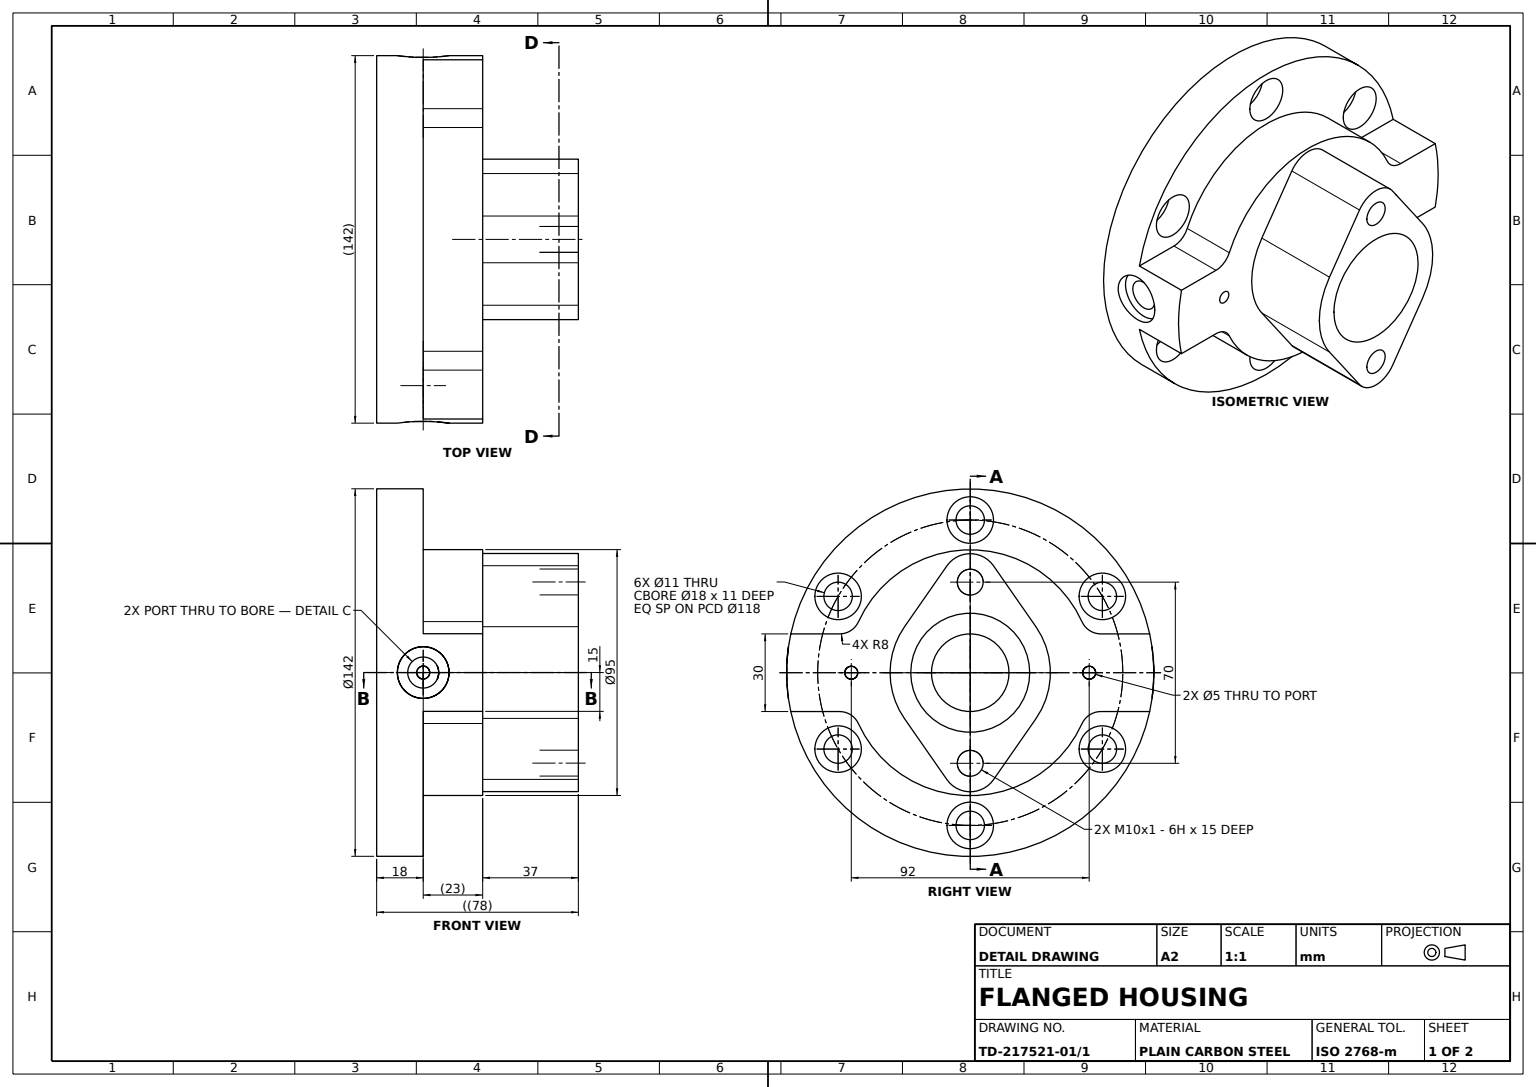
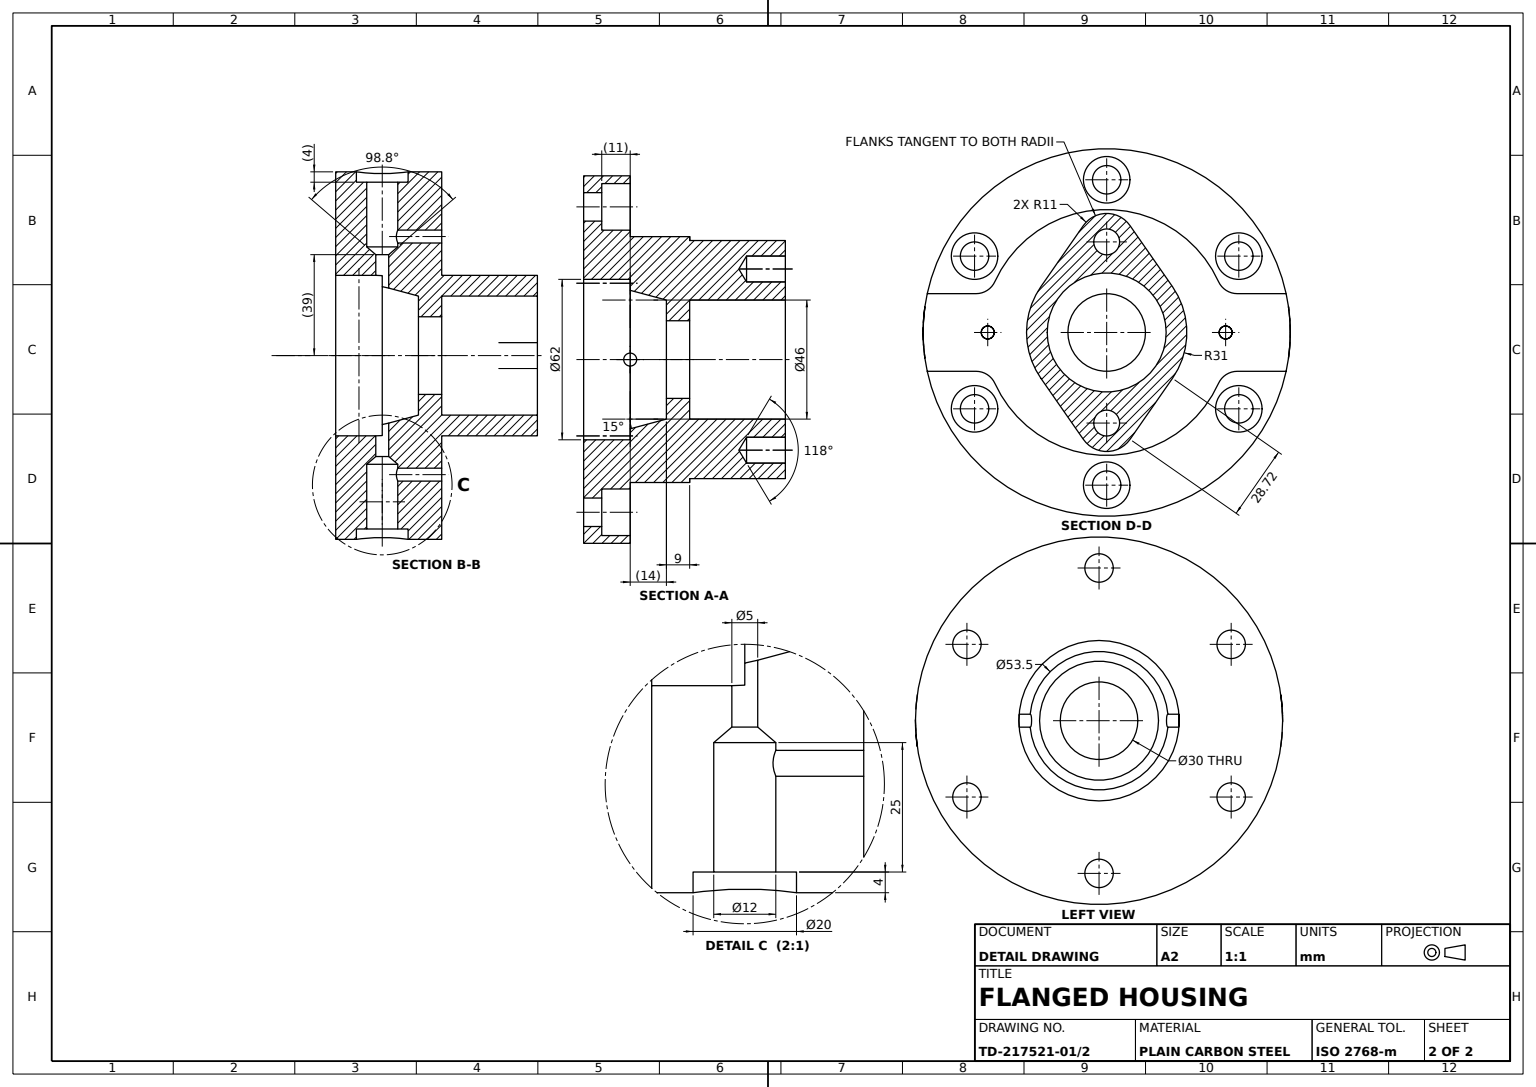
SolidWorks part; units mm, degrees
material "Plain Carbon Steel"
ref_plane "Front Plane" through (0, 0, 0) normal (0, 0, 1) x (1, 0, 0)
ref_plane "Top Plane" through (0, 0, 0) normal (0, 1, 0) x (1, 0, 0)
ref_plane "Right Plane" through (0, 0, 0) normal (1, 0, 0) x (0, 0, -1)
sketch "Base Flange Sketch" plane through (0, 0, 0) normal (0, 0, 1) x (1, 0, 0)
  circle A0 centre (0, 0) radius 71
  dimension "D1" = 142
extrude "Base Flange Ø142" add sketch "Base Flange Sketch" along normal blind 18
sketch "Middle Boss Sketch" plane through (0, 0, 0) normal (0, 0, -1) x (-1, 0, 0)
  line L0 (-81.5219, 0) -> (75.8672, 0) construction
  line L1 (50.5099, 15) -> (69.3974, 15)
  line L2 (50.5099, -15) -> (69.3974, -15)
  line L3 (0, 108.8072) -> (0, -83.8209) construction
  line L4 (-50.5099, -15) -> (-69.3974, -15)
  line L5 (-50.5099, 15) -> (-69.3974, 15)
  arc A0 (43.2292, 19.6847) -> (-43.2292, 19.6847) centre (0, 0) ccw
  arc A1 (69.3974, -15) -> (69.3974, 15) centre (0, 0) ccw
  circle A5 centre (0, 0) radius 71 construction
  arc A6 (-69.3974, 15) -> (-69.3974, -15) centre (0, 0) ccw
  arc A7 (-43.2292, -19.6847) -> (43.2292, -19.6847) centre (0, 0) ccw
  arc A8 (50.5099, -15) -> (43.2292, -19.6847) centre (50.5099, -23) ccw
  arc A9 (50.5099, 15) -> (43.2292, 19.6847) centre (50.5099, 23) cw
  arc A10 (-43.2292, 19.6847) -> (-50.5099, 15) centre (-50.5099, 23) cw
  arc A11 (-50.5099, -15) -> (-43.2292, -19.6847) centre (-50.5099, -23) cw
  point P17 (45.0694, -15)
  point P20 (45.0694, 15)
  point P23 (-45.0694, 15)
  point P26 (-45.0694, -15)
  dimension "D1" = 95
  dimension "D3" = 8
  dimension "D2" = 15
extrude "Middle Boss" add sketch "Middle Boss Sketch" along normal blind 23
sketch "Oval Flange Sketch" plane through (0, 0, -23) normal (0, 0, -1) x (-1, 0, 0)
  line L0 (0, 31.4693) -> (0, -35) construction
  line L1 (-58.0152, 0) -> (50.3973, 0) construction
  line L2 (-9.0272, 41.2857) -> (-25.4402, 17.7143)
  line L3 (9.0272, 41.2857) -> (25.4402, 17.7143)
  line L4 (9.0272, -41.2857) -> (25.4402, -17.7143)
  line L5 (-9.0272, -41.2857) -> (-25.4402, -17.7143)
  circle A1 centre (0, 0) radius 23
  arc A2 (-25.4402, 17.7143) -> (-25.4402, -17.7143) centre (0, 0) ccw
  arc A6 (9.0272, -41.2857) -> (-9.0272, -41.2857) centre (0, -35) cw
  arc A7 (25.4402, -17.7143) -> (25.4402, 17.7143) centre (0, 0) ccw
  arc A8 (9.0272, 41.2857) -> (-9.0272, 41.2857) centre (0, 35) ccw
  dimension "D1" = 62
  dimension "D2" = 46
  dimension "D3" = 70
  dimension "D5" = 28.7228
  dimension "D6" = 11
extrude "Oval Top Flange" add sketch "Oval Flange Sketch" along normal blind 37
sketch "Bolt Hole Position Sketch" plane through (0, 0, 0) normal (0, 0, -1) x (-1, 0, 0)
  line L0 (0, 59) -> (0, -59) construction
  dimension "D1" = 118
  dimension "D2" = 59
hole_wizard "Counterbored Bolt Hole M10" positions "Sketch7" profile "Sketch8" counterbore size "M10" standard "ANSI Metric" end condition through all
sketch "Sketch7" plane through (0, 0, 0) normal (0, 0, -1) x (-1, 0, 0)
  point P0 (0, -59)
sketch "Sketch8" plane through (0, -59, 0) normal (1, 0, 0) x (0, 1, 0)
  line L0 (0, 0) -> (0, 18)
  line L1 (0, 18) -> (5.5, 18)
  line L3 (5.5, 18) -> (5.5, 11)
  line L4 (5.5, 11) -> (9, 11)
  line L5 (9, 11) -> (9, 0)
  line L7 (9, 0) -> (0, 0)
  line L11 (0, -6.35) -> (0, 107.95) construction
  dimension "Thru Hole Dia." = 11
  dimension "Thru Hole Depth" = 18
  dimension "C'Bore Dia." = 18
  dimension "C'Bore Depth" = 11
pattern_circular "Bolt Hole Pattern 6x" count 6 over 360 about axis through (0, 0, 0) along (0, 0, 1) of "Counterbored Bolt Hole M10"
sketch "Central Bore Profile" plane through (0, 0, 0) normal (0, 1, 0) x (1, 0, 0)
  line L0 (0, 90.8034) -> (0, -64.7959) construction
  line L1 (109.8503, 0) -> (26.7513, 0) construction
  line L2 (0, 23) -> (0, -18)
  line L3 (31, 0) -> (26.7513, 0)
  line L4 (31, 0) -> (31, -18)
  line L5 (31, -18) -> (0, -18)
  line L7 (23, 14) -> (26.7513, 0)
  line L8 (23, 14) -> (15, 14)
  line L9 (15, 14) -> (15, 23)
  line L10 (43.2292, 23) -> (-43.2292, 23) construction
  line L11 (15, 23) -> (0, 23)
  dimension "D1" = 18
  dimension "D2" = 31
  dimension "D3" = 23
  dimension "D6" = 15
  dimension "D7" = 9
  dimension "D8" = 15
revolve "Central Bore" cut sketch "Central Bore Profile" angle 360 about L2
sketch "Side Port Profile" plane through (0, 0, 0) normal (0, 1, 0) x (1, 0, 0)
  line L0 (0, 23) -> (0, -18) construction
  line L2 (9.0272, 23) -> (-9.0272, 23) construction
  line L4 (-71, -18) -> (71, -18) construction
  line L5 (-79.2961, 0) -> (15.2993, 0) construction
  line L6 (71, 0) -> (71, -10)
  line L7 (71, -18) -> (71, 23) construction
  line L10 (67, -10) -> (71, -10)
  line L11 (71, 0) -> (88.3372, 0) construction
  line L12 (42, -6) -> (67, -6)
  line L16 (15.2993, 0) -> (71, 0)
  line L18 (39, -2.5) -> (42, -6)
  line L20 (67, -6) -> (67, -10)
  line L21 (39, -2.5) -> (15.2993, -2.5)
  line L22 (15.2993, -2.5) -> (15.2993, 0)
  dimension "D1" = 15.2993
  dimension "D2" = 10
  dimension "D4" = 39
  dimension "D6" = 6
  dimension "D9" = 2.5
  dimension "D3" = 25
revolve "Side Port" cut sketch "Side Port Profile" angle 360 about L5
mirror "Side Port Mirror" about plane through (0, 0, 0) normal (1, 0, 0) of "Side Port"
hole_wizard "Clearance Hole M5" positions "Sketch17" profile "Sketch16" hole size "M5" standard "ANSI Metric"
sketch "Sketch17" plane through (0, 0, -23) normal (0, 0, -1) x (-1, 0, 0)
  point P0 (-46, 0)
  point P1 (46, 0)
  dimension "D1" = 92
  dimension "D2" = 46
sketch "Sketch16" plane through (46, 0, -23) normal (1, 0, 0) x (0, 1, 0)
  line L0 (0, 0) -> (0, 19.5022)
  line L1 (0, 19.5022) -> (2.5, 18)
  line L2 (2.5, 18) -> (2.5, 0)
  line L5 (2.5, 0) -> (0, 0)
  line L10 (0, 19.5022) -> (-2.5, 18) construction
  line L11 (0, -6.35) -> (0, 107.95) construction
  dimension "Hole Dia." = 5
  dimension "Hole Depth" = 18
  dimension "Drill Angle" = 118
hole_wizard "Tapped Hole M10x1.0" positions "Sketch18" profile "Sketch19" tap size "M10x1.0" standard "ANSI Metric"
sketch "Sketch18" plane through (0, 0, -60) normal (0, 0, -1) x (-1, 0, 0)
  point P0 (0, -35)
  point P2 (0, 35)
  dimension "D1" = 35
  dimension "D2" = 35
sketch "Sketch19" plane through (0, -35, -60) normal (1, 0, 0) x (0, 1, 0)
  line L0 (0, 0) -> (0, 18.0043)
  line L1 (0, 18.0043) -> (5, 15)
  line L2 (5, 15) -> (5, 0)
  line L5 (5, 0) -> (0, 0)
  line L10 (0, 18.0043) -> (-5, 15) construction
  line L11 (0, -6.35) -> (0, 107.95) construction
  dimension "Tap Drill Dia." = 10
  dimension "Tap Drill Depth" = 15
  dimension "Drill Angle" = 118
